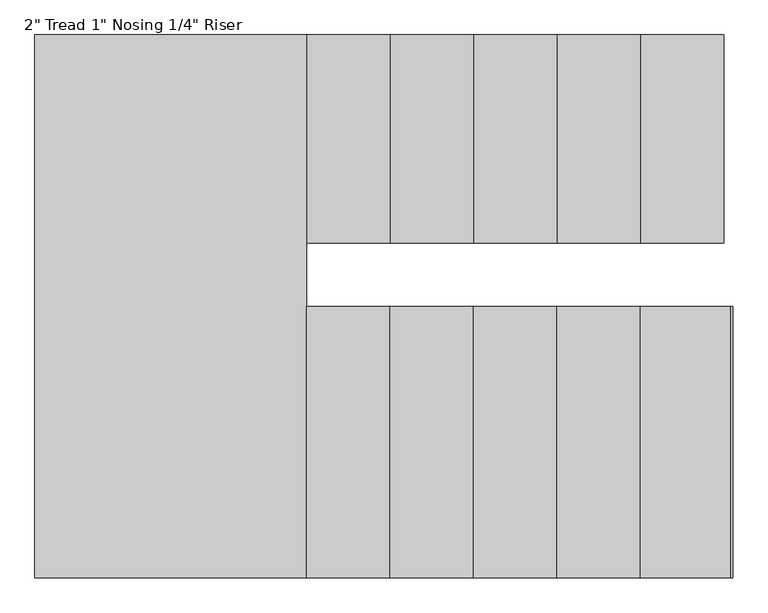
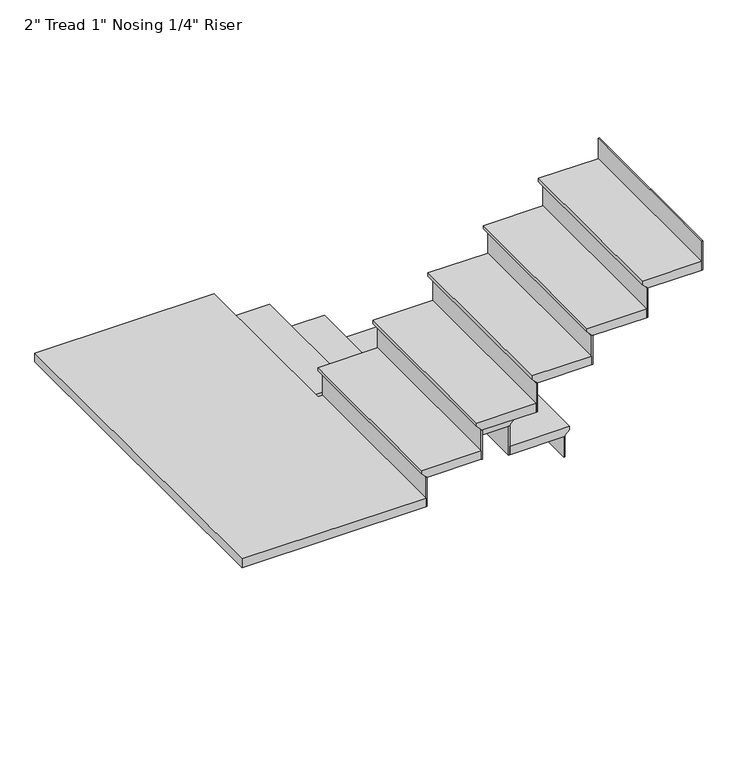
"""IFC4 building model written with IfcOpenShell, lengths in millimetres: stair flight geometry."""

from ifc_helpers import new_model, si_unit, origin, place, context, project, spatial, faceted_brep, source, transform, mapped, element, save


def stair_flight_c1fd4bb9(model_context):
    return source(origin(), model_context, "Body", "Brep", [
        faceted_brep([(-3084.0415084, -317.1427733, 150.2833333), (-3084.0415084, -317.1427733, 169.3333333), (-3084.0415084, -1076.6758739, 169.3333333), (-3084.0415084, -1076.6758739, 150.2833333), (-3109.4415084, -317.1427733, 124.8833333), (-3109.4415084, -1076.6758739, 124.8833333), (-3414.2415084, -317.1427733, 169.3333333), (-3414.2415084, -1076.6758739, 169.3333333), (-3109.4415084, -1076.6758739, 118.5333333), (-3414.2415084, -1076.6758739, 118.5333333), (-3414.2415084, -317.1427733, 118.5333333), (-3109.4415084, -317.1427733, 118.5333333)], [[[0, 1, 2, 3]], [[4, 0, 3, 5]], [[2, 1, 6, 7]], [[8, 9, 10, 11]], [[2, 7, 9, 8, 5, 3]], [[8, 11, 4, 5]], [[6, 1, 0, 4, 11, 10]], [[7, 6, 10, 9]]]),
        faceted_brep([(-3109.4415084, -317.1427733, 118.5333333), (-3109.4415084, -317.1427733, 0.0), (-3115.7915084, -317.1427733, 0.0), (-3115.7915084, -317.1427733, 118.5333333), (-3109.4415084, -1076.6758739, 118.5333333), (-3115.7915084, -1076.6758739, 118.5333333), (-3115.7915084, -1076.6758739, 0.0), (-3109.4415084, -1076.6758739, 0.0)], [[[0, 1, 2, 3]], [[4, 5, 6, 7]], [[1, 0, 4, 7]], [[2, 1, 7, 6]], [[3, 2, 6, 5]], [[0, 3, 5, 4]]]),
        faceted_brep([(-3414.2415084, -317.1427733, 287.8666667), (-3414.2415084, -317.1427733, 118.5333333), (-3420.5915084, -317.1427733, 118.5333333), (-3420.5915084, -317.1427733, 287.8666667), (-3414.2415084, -1076.6758739, 287.8666667), (-3420.5915084, -1076.6758739, 287.8666667), (-3420.5915084, -1076.6758739, 118.5333333), (-3414.2415084, -1076.6758739, 118.5333333)], [[[0, 1, 2, 3]], [[4, 5, 6, 7]], [[1, 0, 4, 7]], [[2, 1, 7, 6]], [[3, 2, 6, 5]], [[0, 3, 5, 4]]]),
        faceted_brep([(-3388.8415084, -1076.6758739, 338.6666667), (-3388.8415084, -317.1427733, 338.6666667), (-3719.0415084, -317.1427733, 338.6666667), (-3719.0415084, -1076.6758739, 338.6666667), (-3414.2415084, -1076.6758739, 287.8666667), (-3719.0415084, -1076.6758739, 287.8666667), (-3719.0415084, -317.1427733, 287.8666667), (-3414.2415084, -317.1427733, 287.8666667), (-3414.2415084, -1076.6758739, 294.2166667), (-3388.8415084, -1076.6758739, 319.6166667), (-3414.2415084, -317.1427733, 294.2166667), (-3388.8415084, -317.1427733, 319.6166667)], [[[0, 1, 2, 3]], [[4, 5, 6, 7]], [[0, 3, 5, 4, 8, 9]], [[4, 7, 10, 8]], [[2, 1, 11, 10, 7, 6]], [[3, 2, 6, 5]], [[11, 1, 0, 9]], [[10, 11, 9, 8]]]),
        faceted_brep([(-3719.0415084, -317.1427733, 457.2), (-3719.0415084, -317.1427733, 287.8666667), (-3725.3915084, -317.1427733, 287.8666667), (-3725.3915084, -317.1427733, 457.2), (-3719.0415084, -1076.6758739, 457.2), (-3725.3915084, -1076.6758739, 457.2), (-3725.3915084, -1076.6758739, 287.8666667), (-3719.0415084, -1076.6758739, 287.8666667)], [[[0, 1, 2, 3]], [[4, 5, 6, 7]], [[1, 0, 4, 7]], [[2, 1, 7, 6]], [[3, 2, 6, 5]], [[0, 3, 5, 4]]]),
        faceted_brep([(-3693.6415084, -1076.6758739, 508.0), (-3693.6415084, -317.1427733, 508.0), (-4023.8415084, -317.1427733, 508.0), (-4023.8415084, -1076.6758739, 508.0), (-3719.0415084, -1076.6758739, 457.2), (-4023.8415084, -1076.6758739, 457.2), (-4023.8415084, -317.1427733, 457.2), (-3719.0415084, -317.1427733, 457.2), (-3719.0415084, -1076.6758739, 463.55), (-3693.6415084, -1076.6758739, 488.95), (-3719.0415084, -317.1427733, 463.55), (-3693.6415084, -317.1427733, 488.95)], [[[0, 1, 2, 3]], [[4, 5, 6, 7]], [[0, 3, 5, 4, 8, 9]], [[4, 7, 10, 8]], [[2, 1, 11, 10, 7, 6]], [[3, 2, 6, 5]], [[11, 1, 0, 9]], [[10, 11, 9, 8]]]),
        faceted_brep([(-4023.8415084, -317.1427733, 626.5333333), (-4023.8415084, -317.1427733, 457.2), (-4030.1915084, -317.1427733, 457.2), (-4030.1915084, -317.1427733, 626.5333333), (-4023.8415084, -1076.6758739, 626.5333333), (-4030.1915084, -1076.6758739, 626.5333333), (-4030.1915084, -1076.6758739, 457.2), (-4023.8415084, -1076.6758739, 457.2)], [[[0, 1, 2, 3]], [[4, 5, 6, 7]], [[1, 0, 4, 7]], [[2, 1, 7, 6]], [[3, 2, 6, 5]], [[0, 3, 5, 4]]]),
        faceted_brep([(-3998.4415084, -1076.6758739, 677.3333333), (-3998.4415084, -317.1427733, 677.3333333), (-4328.6415084, -317.1427733, 677.3333333), (-4328.6415084, -1076.6758739, 677.3333333), (-4023.8415084, -1076.6758739, 626.5333333), (-4328.6415084, -1076.6758739, 626.5333333), (-4328.6415084, -317.1427733, 626.5333333), (-4023.8415084, -317.1427733, 626.5333333), (-4023.8415084, -1076.6758739, 632.8833333), (-3998.4415084, -1076.6758739, 658.2833333), (-4023.8415084, -317.1427733, 632.8833333), (-3998.4415084, -317.1427733, 658.2833333)], [[[0, 1, 2, 3]], [[4, 5, 6, 7]], [[0, 3, 5, 4, 8, 9]], [[4, 7, 10, 8]], [[2, 1, 11, 10, 7, 6]], [[3, 2, 6, 5]], [[11, 1, 0, 9]], [[10, 11, 9, 8]]]),
        faceted_brep([(-4328.6415084, -317.1427733, 795.8666667), (-4328.6415084, -317.1427733, 626.5333333), (-4334.9915084, -317.1427733, 626.5333333), (-4334.9915084, -317.1427733, 795.8666667), (-4328.6415084, -1076.6758739, 795.8666667), (-4334.9915084, -1076.6758739, 795.8666667), (-4334.9915084, -1076.6758739, 626.5333333), (-4328.6415084, -1076.6758739, 626.5333333)], [[[0, 1, 2, 3]], [[4, 5, 6, 7]], [[1, 0, 4, 7]], [[2, 1, 7, 6]], [[3, 2, 6, 5]], [[0, 3, 5, 4]]]),
        faceted_brep([(-4303.2415084, -1076.6758739, 846.6666667), (-4303.2415084, -317.1427733, 846.6666667), (-4633.4415084, -317.1427733, 846.6666667), (-4633.4415084, -1076.6758739, 846.6666667), (-4328.6415084, -1076.6758739, 795.8666667), (-4633.4415084, -1076.6758739, 795.8666667), (-4633.4415084, -317.1427733, 795.8666667), (-4328.6415084, -317.1427733, 795.8666667), (-4328.6415084, -1076.6758739, 802.2166667), (-4303.2415084, -1076.6758739, 827.6166667), (-4328.6415084, -317.1427733, 802.2166667), (-4303.2415084, -317.1427733, 827.6166667)], [[[0, 1, 2, 3]], [[4, 5, 6, 7]], [[0, 3, 5, 4, 8, 9]], [[4, 7, 10, 8]], [[2, 1, 11, 10, 7, 6]], [[3, 2, 6, 5]], [[11, 1, 0, 9]], [[10, 11, 9, 8]]]),
        faceted_brep([(-4633.4415084, -317.1427733, 965.2), (-4633.4415084, -317.1427733, 795.8666667), (-4639.7915084, -317.1427733, 795.8666667), (-4639.7915084, -317.1427733, 965.2), (-4633.4415084, -1076.6758739, 965.2), (-4639.7915084, -1076.6758739, 965.2), (-4639.7915084, -1076.6758739, 795.8666667), (-4633.4415084, -1076.6758739, 795.8666667)], [[[0, 1, 2, 3]], [[4, 5, 6, 7]], [[1, 0, 4, 7]], [[2, 1, 7, 6]], [[3, 2, 6, 5]], [[0, 3, 5, 4]]]),
        faceted_brep([(-4582.6415084, -1307.7427733, 1016.0), (-4608.0415084, -1307.7427733, 1016.0), (-4608.0415084, -317.1427733, 1016.0), (-5598.6415084, -317.1427733, 1016.0), (-5598.6415084, -2298.3427733, 1016.0), (-4582.6415084, -2298.3427733, 1016.0), (-4608.0415084, -1307.7427733, 965.2), (-4582.6415084, -1307.7427733, 965.2), (-4582.6415084, -2298.3427733, 965.2), (-5598.6415084, -2298.3427733, 965.2), (-5598.6415084, -317.1427733, 965.2), (-4633.4415084, -317.1427733, 965.2), (-4633.4415084, -1076.6758739, 965.2), (-4608.0415084, -1076.6758739, 965.2), (-4608.0415084, -1076.6758739, 996.95), (-4608.0415084, -317.1427733, 996.95), (-4633.4415084, -1076.6758739, 971.55), (-4633.4415084, -317.1427733, 971.55)], [[[0, 1, 2, 3, 4, 5]], [[6, 7, 8, 9, 10, 11, 12, 13]], [[1, 0, 7, 6]], [[2, 1, 6, 13, 14, 15]], [[13, 12, 16, 14]], [[12, 11, 17, 16]], [[3, 2, 15, 17, 11, 10]], [[4, 3, 10, 9]], [[5, 4, 9, 8]], [[0, 5, 8, 7]], [[17, 15, 14, 16]]]),
        faceted_brep([(-4582.6415084, -2298.3427733, 1134.5333333), (-4582.6415084, -2298.3427733, 965.2), (-4576.2915084, -2298.3427733, 965.2), (-4576.2915084, -2298.3427733, 1134.5333333), (-4582.6415084, -1307.7427733, 1134.5333333), (-4576.2915084, -1307.7427733, 1134.5333333), (-4576.2915084, -1307.7427733, 965.2), (-4582.6415084, -1307.7427733, 965.2)], [[[0, 1, 2, 3]], [[4, 5, 6, 7]], [[1, 0, 4, 7]], [[2, 1, 7, 6]], [[3, 2, 6, 5]], [[0, 3, 5, 4]]]),
        faceted_brep([(-4608.0415084, -1307.7427733, 1185.3333333), (-4608.0415084, -2298.3427733, 1185.3333333), (-4277.8415084, -2298.3427733, 1185.3333333), (-4277.8415084, -1307.7427733, 1185.3333333), (-4582.6415084, -1307.7427733, 1134.5333333), (-4277.8415084, -1307.7427733, 1134.5333333), (-4277.8415084, -2298.3427733, 1134.5333333), (-4582.6415084, -2298.3427733, 1134.5333333), (-4582.6415084, -1307.7427733, 1140.8833333), (-4608.0415084, -1307.7427733, 1166.2833333), (-4582.6415084, -2298.3427733, 1140.8833333), (-4608.0415084, -2298.3427733, 1166.2833333)], [[[0, 1, 2, 3]], [[4, 5, 6, 7]], [[0, 3, 5, 4, 8, 9]], [[4, 7, 10, 8]], [[2, 1, 11, 10, 7, 6]], [[3, 2, 6, 5]], [[11, 1, 0, 9]], [[10, 11, 9, 8]]]),
        faceted_brep([(-4277.8415084, -2298.3427733, 1303.8666667), (-4277.8415084, -2298.3427733, 1134.5333333), (-4271.4915084, -2298.3427733, 1134.5333333), (-4271.4915084, -2298.3427733, 1303.8666667), (-4277.8415084, -1307.7427733, 1303.8666667), (-4271.4915084, -1307.7427733, 1303.8666667), (-4271.4915084, -1307.7427733, 1134.5333333), (-4277.8415084, -1307.7427733, 1134.5333333)], [[[0, 1, 2, 3]], [[4, 5, 6, 7]], [[1, 0, 4, 7]], [[2, 1, 7, 6]], [[3, 2, 6, 5]], [[0, 3, 5, 4]]]),
        faceted_brep([(-4303.2415084, -1307.7427733, 1354.6666667), (-4303.2415084, -2298.3427733, 1354.6666667), (-3973.0415084, -2298.3427733, 1354.6666667), (-3973.0415084, -1307.7427733, 1354.6666667), (-4277.8415084, -1307.7427733, 1303.8666667), (-3973.0415084, -1307.7427733, 1303.8666667), (-3973.0415084, -2298.3427733, 1303.8666667), (-4277.8415084, -2298.3427733, 1303.8666667), (-4277.8415084, -1307.7427733, 1310.2166667), (-4303.2415084, -1307.7427733, 1335.6166667), (-4277.8415084, -2298.3427733, 1310.2166667), (-4303.2415084, -2298.3427733, 1335.6166667)], [[[0, 1, 2, 3]], [[4, 5, 6, 7]], [[0, 3, 5, 4, 8, 9]], [[4, 7, 10, 8]], [[2, 1, 11, 10, 7, 6]], [[3, 2, 6, 5]], [[11, 1, 0, 9]], [[10, 11, 9, 8]]]),
        faceted_brep([(-3973.0415084, -2298.3427733, 1473.2), (-3973.0415084, -2298.3427733, 1303.8666667), (-3966.6915084, -2298.3427733, 1303.8666667), (-3966.6915084, -2298.3427733, 1473.2), (-3973.0415084, -1307.7427733, 1473.2), (-3966.6915084, -1307.7427733, 1473.2), (-3966.6915084, -1307.7427733, 1303.8666667), (-3973.0415084, -1307.7427733, 1303.8666667)], [[[0, 1, 2, 3]], [[4, 5, 6, 7]], [[1, 0, 4, 7]], [[2, 1, 7, 6]], [[3, 2, 6, 5]], [[0, 3, 5, 4]]]),
        faceted_brep([(-3998.4415084, -1307.7427733, 1524.0), (-3998.4415084, -2298.3427733, 1524.0), (-3668.2415084, -2298.3427733, 1524.0), (-3668.2415084, -1307.7427733, 1524.0), (-3973.0415084, -1307.7427733, 1473.2), (-3668.2415084, -1307.7427733, 1473.2), (-3668.2415084, -2298.3427733, 1473.2), (-3973.0415084, -2298.3427733, 1473.2), (-3973.0415084, -1307.7427733, 1479.55), (-3998.4415084, -1307.7427733, 1504.95), (-3973.0415084, -2298.3427733, 1479.55), (-3998.4415084, -2298.3427733, 1504.95)], [[[0, 1, 2, 3]], [[4, 5, 6, 7]], [[0, 3, 5, 4, 8, 9]], [[4, 7, 10, 8]], [[2, 1, 11, 10, 7, 6]], [[3, 2, 6, 5]], [[11, 1, 0, 9]], [[10, 11, 9, 8]]]),
        faceted_brep([(-3668.2415084, -2298.3427733, 1642.5333333), (-3668.2415084, -2298.3427733, 1473.2), (-3661.8915084, -2298.3427733, 1473.2), (-3661.8915084, -2298.3427733, 1642.5333333), (-3668.2415084, -1307.7427733, 1642.5333333), (-3661.8915084, -1307.7427733, 1642.5333333), (-3661.8915084, -1307.7427733, 1473.2), (-3668.2415084, -1307.7427733, 1473.2)], [[[0, 1, 2, 3]], [[4, 5, 6, 7]], [[1, 0, 4, 7]], [[2, 1, 7, 6]], [[3, 2, 6, 5]], [[0, 3, 5, 4]]]),
        faceted_brep([(-3693.6415084, -1307.7427733, 1693.3333333), (-3693.6415084, -2298.3427733, 1693.3333333), (-3363.4415084, -2298.3427733, 1693.3333333), (-3363.4415084, -1307.7427733, 1693.3333333), (-3668.2415084, -1307.7427733, 1642.5333333), (-3363.4415084, -1307.7427733, 1642.5333333), (-3363.4415084, -2298.3427733, 1642.5333333), (-3668.2415084, -2298.3427733, 1642.5333333), (-3668.2415084, -1307.7427733, 1648.8833333), (-3693.6415084, -1307.7427733, 1674.2833333), (-3668.2415084, -2298.3427733, 1648.8833333), (-3693.6415084, -2298.3427733, 1674.2833333)], [[[0, 1, 2, 3]], [[4, 5, 6, 7]], [[0, 3, 5, 4, 8, 9]], [[4, 7, 10, 8]], [[2, 1, 11, 10, 7, 6]], [[3, 2, 6, 5]], [[11, 1, 0, 9]], [[10, 11, 9, 8]]]),
        faceted_brep([(-3363.4415084, -2298.3427733, 1811.8666667), (-3363.4415084, -2298.3427733, 1642.5333333), (-3357.0915084, -2298.3427733, 1642.5333333), (-3357.0915084, -2298.3427733, 1811.8666667), (-3363.4415084, -1307.7427733, 1811.8666667), (-3357.0915084, -1307.7427733, 1811.8666667), (-3357.0915084, -1307.7427733, 1642.5333333), (-3363.4415084, -1307.7427733, 1642.5333333)], [[[0, 1, 2, 3]], [[4, 5, 6, 7]], [[1, 0, 4, 7]], [[2, 1, 7, 6]], [[3, 2, 6, 5]], [[0, 3, 5, 4]]]),
        faceted_brep([(-3058.6415084, -2298.3427733, 1981.2), (-3058.6415084, -2298.3427733, 1811.8666667), (-3052.2915084, -2298.3427733, 1811.8666667), (-3052.2915084, -2298.3427733, 1981.2), (-3058.6415084, -1307.7427733, 1981.2), (-3052.2915084, -1307.7427733, 1981.2), (-3052.2915084, -1307.7427733, 1811.8666667), (-3058.6415084, -1307.7427733, 1811.8666667)], [[[0, 1, 2, 3]], [[4, 5, 6, 7]], [[1, 0, 4, 7]], [[2, 1, 7, 6]], [[3, 2, 6, 5]], [[0, 3, 5, 4]]]),
        faceted_brep([(-3388.8415084, -1307.7427733, 1862.6666667), (-3388.8415084, -2298.3427733, 1862.6666667), (-3058.6415084, -2298.3427733, 1862.6666667), (-3058.6415084, -1307.7427733, 1862.6666667), (-3363.4415084, -1307.7427733, 1811.8666667), (-3058.6415084, -1307.7427733, 1811.8666667), (-3058.6415084, -2298.3427733, 1811.8666667), (-3363.4415084, -2298.3427733, 1811.8666667), (-3363.4415084, -1307.7427733, 1818.2166667), (-3388.8415084, -1307.7427733, 1843.6166667), (-3363.4415084, -2298.3427733, 1818.2166667), (-3388.8415084, -2298.3427733, 1843.6166667)], [[[0, 1, 2, 3]], [[4, 5, 6, 7]], [[0, 3, 5, 4, 8, 9]], [[4, 7, 10, 8]], [[2, 1, 11, 10, 7, 6]], [[3, 2, 6, 5]], [[11, 1, 0, 9]], [[10, 11, 9, 8]]]),
    ])


if __name__ == "__main__":
    model = new_model("IFC4")
    model_context = context("Model", 3, world=origin())
    ifc_project = project(units=[si_unit("LENGTHUNIT", "METRE", prefix="MILLI")], contexts=[model_context])
    site = spatial("IfcSite", under=ifc_project)
    building = spatial("IfcBuilding", under=site)
    placement = place(None, origin())
    stair_flight_shape = stair_flight_c1fd4bb9(model_context)
    element("IfcStairFlight", 1, ObjectType="2\" Tread 1\" Nosing 1/4\" Riser", at=placement, inside=building, context=model_context, shape_type="MappedRepresentation", body=[
        mapped(stair_flight_shape, transform((0.0, 0.0, 0.0), x_axis=(1.0, 0.0, 0.0), y_axis=(0.0, 1.0, 0.0), z_axis=(0.0, 0.0, 1.0))),
    ])
    save(model, "model.ifc")
